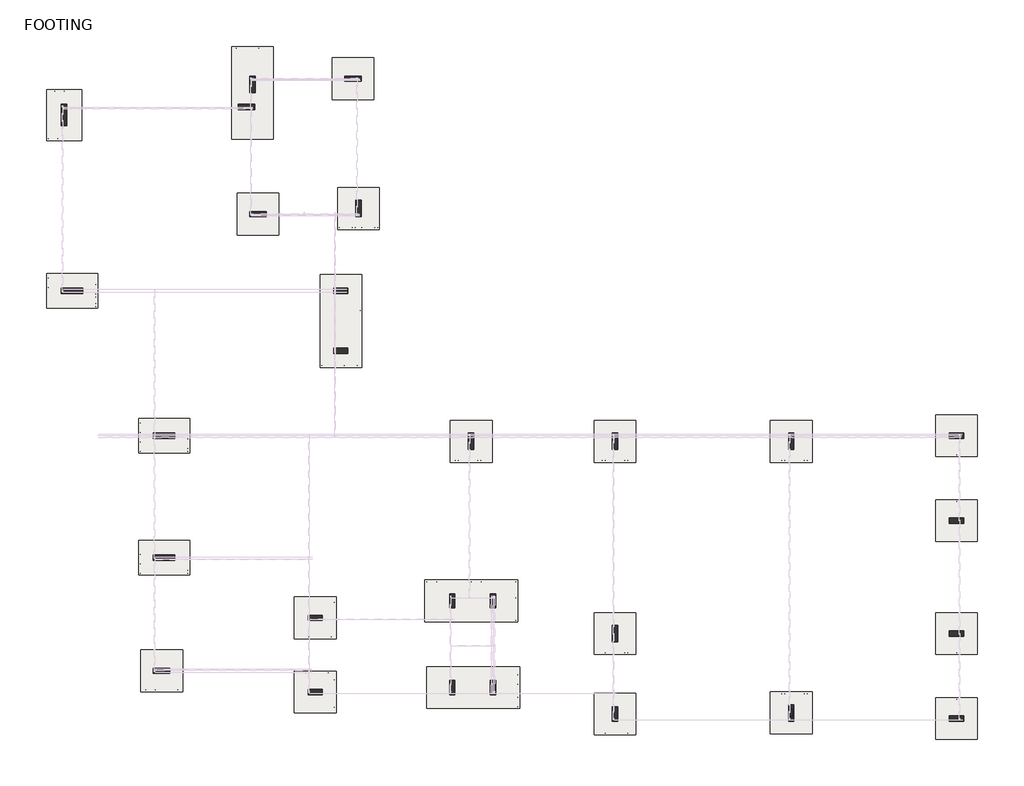
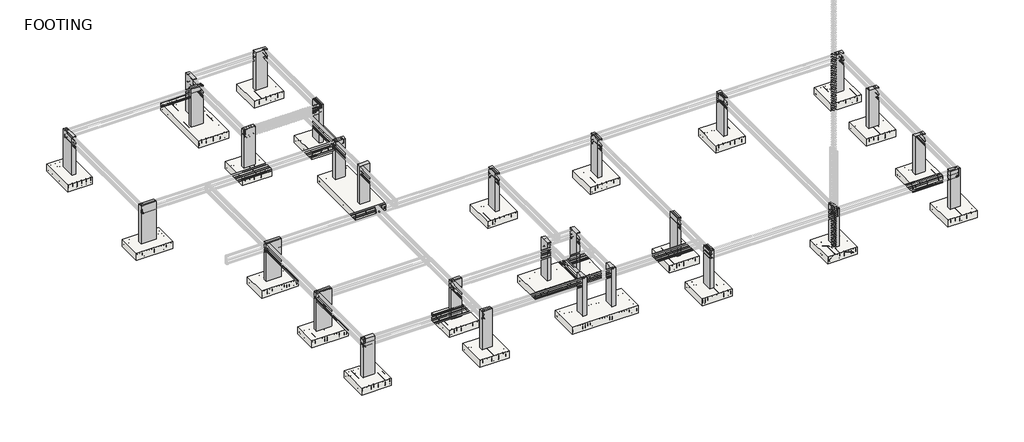
# One storey, part 1 of 12: 28 columns, 24 slabs.
"""IFC4 building model written with IfcOpenShell, lengths in millimetres."""

from ifc_helpers import new_model, si_unit, frame, origin, place, context, project, spatial, polyline, outline, extrude, faceted_brep, transform, mapped, element, save
from components import m_footing_rectangular_e5d4dde8, m_footing_rectangular_b51645d7, m_footing_rectangular_2200_x1500m_x450mm_63325679

model = new_model("IFC4")

# Units and contexts
model_context = context("Model", 3, world=origin())
ifc_project = project(units=[si_unit("LENGTHUNIT", "METRE", prefix="MILLI")], contexts=[model_context])

# Site, building, storey
site = spatial("IfcSite", under=ifc_project)
building = spatial("IfcBuilding", under=site)
storey = spatial("IfcBuildingStorey", under=building, Name="FOOTING", Elevation=-5638.8)

# Columns
placement = place(None, origin())
element("IfcColumn", 1, ObjectType="M_Concrete-Rectangular-Column : 9\" X 24\" C3", at=placement, inside=storey, context=model_context, shape_type="SweptSolid", body=[
    extrude(outline(polyline([(-8729.9501665, -13101.6041655), (-8120.3501665, -13101.6041655), (-8120.3501665, -13330.2041655), (-8729.9501665, -13330.2041655), (-8729.9501665, -13101.6041655)])), frame((0.0, 0.0, -5638.8), z_axis=(0.0, 0.0, 1.0), x_axis=(1.0, 0.0, 0.0)), (0.0, 0.0, 1.0), 2438.4),
])
element("IfcColumn", 2, ObjectType="M_Concrete-Rectangular-Column : 9\" X 24\" C3", at=placement, inside=storey, context=model_context, shape_type="SweptSolid", body=[
    extrude(outline(polyline([(-2633.9501665, -13330.2041655), (-2633.9501665, -12720.6041655), (-2405.3501665, -12720.6041655), (-2405.3501665, -13330.2041655), (-2633.9501665, -13330.2041655)])), frame((0.0, 0.0, -5638.8), z_axis=(0.0, 0.0, 1.0), x_axis=(1.0, 0.0, 0.0)), (0.0, 0.0, 1.0), 2438.4),
])
element("IfcColumn", 3, ObjectType="M_Concrete-Rectangular-Column : 9\" X 24\" C3", at=placement, inside=storey, context=model_context, shape_type="SweptSolid", body=[
    extrude(outline(polyline([(-2633.9501665, -9596.4041655), (-2633.9501665, -8986.8041655), (-2405.3501665, -8986.8041655), (-2405.3501665, -9596.4041655), (-2633.9501665, -9596.4041655)])), frame((0.0, 0.0, -5638.8), z_axis=(0.0, 0.0, 1.0), x_axis=(1.0, 0.0, 0.0)), (0.0, 0.0, 1.0), 2438.4),
])
element("IfcColumn", 4, ObjectType="M_Concrete-Rectangular-Column : 9\" X 24\" C3", at=placement, inside=storey, context=model_context, shape_type="SweptSolid", body=[
    extrude(outline(polyline([(-881.3501665, -9596.4041655), (-881.3501665, -8986.8041655), (-652.7501665, -8986.8041655), (-652.7501665, -9596.4041655), (-881.3501665, -9596.4041655)])), frame((0.0, 0.0, -5638.8), z_axis=(0.0, 0.0, 1.0), x_axis=(1.0, 0.0, 0.0)), (0.0, 0.0, 1.0), 2438.4),
])
element("IfcColumn", 5, ObjectType="M_Concrete-Rectangular-Column : 9\" X 24\" C3", at=placement, inside=storey, context=model_context, shape_type="SweptSolid", body=[
    extrude(outline(polyline([(19514.8498335, -14473.2041655), (18905.2498335, -14473.2041655), (18905.2498335, -14244.6041655), (19514.8498335, -14244.6041655), (19514.8498335, -14473.2041655)])), frame((0.0, 0.0, -5638.8), z_axis=(0.0, 0.0, 1.0), x_axis=(1.0, 0.0, 0.0)), (0.0, 0.0, 1.0), 2438.4),
])
element("IfcColumn", 6, ObjectType="M_Concrete-Rectangular-Column : 9\" X 24\" C3", at=placement, inside=storey, context=model_context, shape_type="Brep", body=[
    faceted_brep([(19514.8498335, -10815.6041655, -5638.8), (18905.2498335, -10815.6041655, -5638.8), (18905.2498335, -10587.0041655, -5638.8), (19514.8498335, -10587.0041655, -5638.8), (19514.8498335, -10815.6041655, -3200.4), (19286.2498335, -10815.6041655, -3200.4), (18905.2498335, -10815.6041655, -3200.4), (19514.8498335, -10815.6041655, -3800.4), (18905.2498335, -10587.0041655, -3200.4), (19286.2498335, -10587.0041655, -3200.4), (19514.8498335, -10587.0041655, -3200.4), (19514.8498335, -10587.0041655, -3800.4)], [[[0, 1, 2, 3]], [[4, 5, 6, 1, 0, 7]], [[6, 8, 2, 1]], [[8, 9, 10, 11, 3, 2]], [[10, 4, 7, 0, 3, 11]], [[4, 10, 9, 8, 6, 5]]]),
])
element("IfcColumn", 7, ObjectType="M_Concrete-Rectangular-Column : 9\" X 24\" C3", at=placement, inside=storey, context=model_context, shape_type="Brep", body=[
    faceted_brep([(19514.8498335, -5938.8041655, -5638.8), (18905.2498335, -5938.8041655, -5638.8), (18905.2498335, -5710.2041655, -5638.8), (19514.8498335, -5710.2041655, -5638.8), (19514.8498335, -5938.8041655, -3200.4), (19286.2498335, -5938.8041655, -3200.4), (18905.2498335, -5938.8041655, -3200.4), (19514.8498335, -5938.8041655, -3800.4), (18905.2498335, -5710.2041655, -3200.4), (19286.2498335, -5710.2041655, -3200.4), (19514.8498335, -5710.2041655, -3200.4), (19514.8498335, -5710.2041655, -3800.4)], [[[0, 1, 2, 3]], [[4, 5, 6, 1, 0, 7]], [[6, 8, 2, 1]], [[8, 9, 10, 11, 3, 2]], [[10, 4, 7, 0, 3, 11]], [[4, 10, 9, 8, 6, 5]]]),
])
element("IfcColumn", 8, ObjectType="M_Concrete-Rectangular-Column : 9\" X 24\" C3", at=placement, inside=storey, context=model_context, shape_type="SweptSolid", body=[
    extrude(outline(polyline([(19514.8498335, -2281.2041655), (18905.2498335, -2281.2041655), (18905.2498335, -2052.6041655), (19514.8498335, -2052.6041655), (19514.8498335, -2281.2041655)])), frame((0.0, 0.0, -5638.8), z_axis=(0.0, 0.0, 1.0), x_axis=(1.0, 0.0, 0.0)), (0.0, 0.0, 1.0), 2438.4),
])
element("IfcColumn", 9, ObjectType="M_Concrete-Rectangular-Column : 9\" X 24\" C3", at=placement, inside=storey, context=model_context, shape_type="SweptSolid", body=[
    extrude(outline(polyline([(-7015.4501665, 3967.1958345), (-7625.0501665, 3967.1958345), (-7625.0501665, 4195.7958345), (-7015.4501665, 4195.7958345), (-7015.4501665, 3967.1958345)])), frame((0.0, 0.0, -5638.8), z_axis=(0.0, 0.0, 1.0), x_axis=(1.0, 0.0, 0.0)), (0.0, 0.0, 1.0), 2438.4),
])
element("IfcColumn", 10, ObjectType="M_Concrete-Rectangular-Column : 9\" X 24\" C3", at=placement, inside=storey, context=model_context, shape_type="Brep", body=[
    faceted_brep([(-7015.4501665, 1376.3958345, -5638.8), (-7625.0501665, 1376.3958345, -5638.8), (-7625.0501665, 1604.9958345, -5638.8), (-7015.4501665, 1604.9958345, -5638.8), (-7015.4501665, 1376.3958345, -3200.4), (-7396.4501665, 1376.3958345, -3200.4), (-7625.0501665, 1376.3958345, -3200.4), (-7625.0501665, 1376.3958345, -3800.4), (-7625.0501665, 1604.9958345, -3200.4), (-7625.0501665, 1604.9958345, -3800.4), (-7396.4501665, 1604.9958345, -3200.4), (-7015.4501665, 1604.9958345, -3200.4)], [[[0, 1, 2, 3]], [[4, 5, 6, 7, 1, 0]], [[6, 8, 9, 2, 1, 7]], [[8, 10, 11, 3, 2, 9]], [[11, 4, 0, 3]], [[4, 11, 10, 8, 6, 5]]]),
])
element("IfcColumn", 11, ObjectType="M_Concrete-Rectangular-Column : 9\" X 24\" C3", at=placement, inside=storey, context=model_context, shape_type="SweptSolid", body=[
    extrude(outline(polyline([(-8729.9501665, -9901.2041655), (-8120.3501665, -9901.2041655), (-8120.3501665, -10129.8041655), (-8729.9501665, -10129.8041655), (-8729.9501665, -9901.2041655)])), frame((0.0, 0.0, -5638.8), z_axis=(0.0, 0.0, 1.0), x_axis=(1.0, 0.0, 0.0)), (0.0, 0.0, 1.0), 2438.4),
])
element("IfcColumn", 12, ObjectType="M_Concrete-Rectangular-Column : 9\" X 24\" C3", at=placement, inside=storey, context=model_context, shape_type="SweptSolid", body=[
    extrude(outline(polyline([(-652.7501665, -12720.6041655), (-652.7501665, -13330.2041655), (-881.3501665, -13330.2041655), (-881.3501665, -12720.6041655), (-652.7501665, -12720.6041655)])), frame((0.0, 0.0, -5638.8), z_axis=(0.0, 0.0, 1.0), x_axis=(1.0, 0.0, 0.0)), (0.0, 0.0, 1.0), 2438.4),
])
element("IfcColumn", 13, ObjectType="M_Concrete-Rectangular-Column : 9\" X 24\" C3", at=placement, inside=storey, context=model_context, shape_type="SweptSolid", body=[
    extrude(outline(polyline([(4605.0498335, -13863.6041655), (4605.0498335, -14473.2041655), (4376.4498335, -14473.2041655), (4376.4498335, -13863.6041655), (4605.0498335, -13863.6041655)])), frame((0.0, 0.0, -5638.8), z_axis=(0.0, 0.0, 1.0), x_axis=(1.0, 0.0, 0.0)), (0.0, 0.0, 1.0), 2438.4),
])
element("IfcColumn", 14, ObjectType="M_Concrete-Rectangular-Column : 9\" X 28\" C2", at=placement, inside=storey, context=model_context, shape_type="SweptSolid", body=[
    extrude(outline(polyline([(-15397.4501665, -12187.2041655), (-14686.2501665, -12187.2041655), (-14686.2501665, -12415.8041655), (-15397.4501665, -12415.8041655), (-15397.4501665, -12187.2041655)])), frame((0.0, 0.0, -5638.8), z_axis=(0.0, 0.0, 1.0), x_axis=(1.0, 0.0, 0.0)), (0.0, 0.0, 1.0), 2438.4),
])
element("IfcColumn", 15, ObjectType="M_Concrete-Rectangular-Column : 9\" X 28\" C2", at=placement, inside=storey, context=model_context, shape_type="Brep", body=[
    faceted_brep([(4376.4498335, -11056.9041655, -5638.8), (4376.4498335, -10345.7041655, -5638.8), (4605.0498335, -10345.7041655, -5638.8), (4605.0498335, -11056.9041655, -5638.8), (4376.4498335, -11056.9041655, -3200.4), (4376.4498335, -10345.7041655, -3200.4), (4376.4498335, -10345.7041655, -3800.4), (4376.4498335, -11056.9041655, -3800.4), (4605.0498335, -10345.7041655, -3200.4), (4605.0498335, -10345.7041655, -3800.4), (4605.0498335, -11056.9041655, -3200.4), (4605.0498335, -11056.9041655, -3800.4)], [[[0, 1, 2, 3]], [[4, 5, 6, 1, 0, 7]], [[5, 8, 9, 2, 1, 6]], [[8, 10, 11, 3, 2, 9]], [[10, 4, 7, 0, 3, 11]], [[4, 10, 8, 5]]]),
])
element("IfcColumn", 16, ObjectType="M_Concrete-Rectangular-Column : 9\" X 28\" C2", at=placement, inside=storey, context=model_context, shape_type="Brep", body=[
    faceted_brep([(11971.0498335, -14473.2041655, -5638.8), (11971.0498335, -13762.0041655, -5638.8), (12199.6498335, -13762.0041655, -5638.8), (12199.6498335, -14473.2041655, -5638.8), (11971.0498335, -14473.2041655, -3200.4), (11971.0498335, -14244.6041655, -3200.4), (11971.0498335, -13762.0041655, -3200.4), (11971.0498335, -14473.2041655, -3800.4), (12199.6498335, -13762.0041655, -3200.4), (12199.6498335, -14244.6041655, -3200.4), (12199.6498335, -14473.2041655, -3200.4), (12199.6498335, -14473.2041655, -3800.4)], [[[0, 1, 2, 3]], [[4, 5, 6, 1, 0, 7]], [[6, 8, 2, 1]], [[8, 9, 10, 11, 3, 2]], [[10, 4, 7, 0, 3, 11]], [[4, 10, 9, 8, 6, 5]]]),
])
element("IfcColumn", 17, ObjectType="M_Concrete-Rectangular-Column : 9\" X 28\" C2", at=placement, inside=storey, context=model_context, shape_type="Brep", body=[
    faceted_brep([(12199.6498335, -2052.6041655, -5638.8), (12199.6498335, -2763.8041655, -5638.8), (11971.0498335, -2763.8041655, -5638.8), (11971.0498335, -2052.6041655, -5638.8), (12199.6498335, -2052.6041655, -3200.4), (12199.6498335, -2281.2041655, -3200.4), (12199.6498335, -2763.8041655, -3200.4), (12199.6498335, -2052.6041655, -3800.4), (11971.0498335, -2763.8041655, -3200.4), (11971.0498335, -2281.2041655, -3200.4), (11971.0498335, -2052.6041655, -3200.4), (11971.0498335, -2052.6041655, -3800.4)], [[[0, 1, 2, 3]], [[4, 5, 6, 1, 0, 7]], [[6, 8, 2, 1]], [[8, 9, 10, 11, 3, 2]], [[10, 4, 7, 0, 3, 11]], [[4, 10, 9, 8, 6, 5]]]),
])
element("IfcColumn", 18, ObjectType="M_Concrete-Rectangular-Column : 9\" X 28\" C2", at=placement, inside=storey, context=model_context, shape_type="Brep", body=[
    faceted_brep([(4605.0498335, -2052.6041655, -5638.8), (4605.0498335, -2763.8041655, -5638.8), (4376.4498335, -2763.8041655, -5638.8), (4376.4498335, -2052.6041655, -5638.8), (4605.0498335, -2052.6041655, -3200.4), (4605.0498335, -2281.2041655, -3200.4), (4605.0498335, -2763.8041655, -3200.4), (4605.0498335, -2052.6041655, -3800.4), (4376.4498335, -2763.8041655, -3200.4), (4376.4498335, -2281.2041655, -3200.4), (4376.4498335, -2052.6041655, -3200.4), (4376.4498335, -2052.6041655, -3800.4)], [[[0, 1, 2, 3]], [[4, 5, 6, 1, 0, 7]], [[6, 8, 2, 1]], [[8, 9, 10, 11, 3, 2]], [[10, 4, 7, 0, 3, 11]], [[4, 10, 9, 8, 6, 5]]]),
])
element("IfcColumn", 19, ObjectType="M_Concrete-Rectangular-Column : 9\" X 28\" C2", at=placement, inside=storey, context=model_context, shape_type="Brep", body=[
    faceted_brep([(-1592.5501665, -2052.6041655, -5638.8), (-1592.5501665, -2763.8041655, -5638.8), (-1821.1501665, -2763.8041655, -5638.8), (-1821.1501665, -2052.6041655, -5638.8), (-1592.5501665, -2052.6041655, -3200.4), (-1592.5501665, -2281.2041655, -3200.4), (-1592.5501665, -2763.8041655, -3200.4), (-1592.5501665, -2052.6041655, -3800.4), (-1821.1501665, -2763.8041655, -3200.4), (-1821.1501665, -2281.2041655, -3200.4), (-1821.1501665, -2052.6041655, -3200.4), (-1821.1501665, -2052.6041655, -3800.4)], [[[0, 1, 2, 3]], [[4, 5, 6, 1, 0, 7]], [[6, 8, 2, 1]], [[8, 9, 10, 11, 3, 2]], [[10, 4, 7, 0, 3, 11]], [[4, 10, 9, 8, 6, 5]]]),
])
element("IfcColumn", 20, ObjectType="M_Concrete-Rectangular-Column : 9\" X 28\" C2", at=placement, inside=storey, context=model_context, shape_type="SweptSolid", body=[
    extrude(outline(polyline([(-11244.5501665, 7503.5858661), (-10533.3501665, 7503.5858661), (-10533.3501665, 7274.9858661), (-11244.5501665, 7274.9858661), (-11244.5501665, 7503.5858661)])), frame((0.0, 0.0, -5638.8), z_axis=(0.0, 0.0, 1.0), x_axis=(1.0, 0.0, 0.0)), (0.0, 0.0, 1.0), 2438.4),
])
element("IfcColumn", 21, ObjectType="M_Concrete-Rectangular-Column : 9\" X 28\" C2", at=placement, inside=storey, context=model_context, shape_type="SweptSolid", body=[
    extrude(outline(polyline([(-6672.5501665, 7274.9858661), (-6672.5501665, 7986.1858661), (-6443.9501665, 7986.1858661), (-6443.9501665, 7274.9858661), (-6672.5501665, 7274.9858661)])), frame((0.0, 0.0, -5638.8), z_axis=(0.0, 0.0, 1.0), x_axis=(1.0, 0.0, 0.0)), (0.0, 0.0, 1.0), 2438.4),
])
element("IfcColumn", 22, ObjectType="M_Concrete-Rectangular-Column : 9\" X 28\" C2", at=placement, inside=storey, context=model_context, shape_type="Brep", body=[
    faceted_brep([(-11028.6501665, 11891.9958345, -5638.8), (-11739.8501665, 11891.9958345, -5638.8), (-11739.8501665, 12120.5958345, -5638.8), (-11028.6501665, 12120.5958345, -5638.8), (-11028.6501665, 11891.9958345, -3200.4), (-11244.5501665, 11891.9958345, -3200.4), (-11739.8501665, 11891.9958345, -3200.4), (-11028.6501665, 11891.9958345, -3800.4), (-11739.8501665, 12120.5958345, -3200.4), (-11244.5501665, 12120.5958345, -3200.4), (-11028.6501665, 12120.5958345, -3200.4), (-11028.6501665, 12120.5958345, -3800.4)], [[[0, 1, 2, 3]], [[4, 5, 6, 1, 0, 7]], [[6, 8, 2, 1]], [[8, 9, 10, 11, 3, 2]], [[10, 4, 7, 0, 3, 11]], [[4, 10, 9, 8, 6, 5]]]),
])
element("IfcColumn", 23, ObjectType="M_Concrete-Rectangular-Column : 9\" X 28\" C2", at=placement, inside=storey, context=model_context, shape_type="SweptSolid", body=[
    extrude(outline(polyline([(-11015.9501665, 13339.7958345), (-11015.9501665, 12628.5958345), (-11244.5501665, 12628.5958345), (-11244.5501665, 13339.7958345), (-11015.9501665, 13339.7958345)])), frame((0.0, 0.0, -5638.8), z_axis=(0.0, 0.0, 1.0), x_axis=(1.0, 0.0, 0.0)), (0.0, 0.0, 1.0), 2438.4),
])
element("IfcColumn", 24, ObjectType="M_Concrete-Rectangular-Column : 9\" X 28\" C2", at=placement, inside=storey, context=model_context, shape_type="SweptSolid", body=[
    extrude(outline(polyline([(-7155.1501665, 13339.7958345), (-6443.9501665, 13339.7958345), (-6443.9501665, 13111.1958345), (-7155.1501665, 13111.1958345), (-7155.1501665, 13339.7958345)])), frame((0.0, 0.0, -5638.8), z_axis=(0.0, 0.0, 1.0), x_axis=(1.0, 0.0, 0.0)), (0.0, 0.0, 1.0), 2438.4),
])
element("IfcColumn", 25, ObjectType="M_Concrete-Rectangular-Column : 9\" X 36\" C1", at=placement, inside=storey, context=model_context, shape_type="SweptSolid", body=[
    extrude(outline(polyline([(-19131.2501665, 12120.5958345), (-19131.2501665, 11206.1958345), (-19359.8501665, 11206.1958345), (-19359.8501665, 12120.5958345), (-19131.2501665, 12120.5958345)])), frame((0.0, 0.0, -5638.8), z_axis=(0.0, 0.0, 1.0), x_axis=(1.0, 0.0, 0.0)), (0.0, 0.0, 1.0), 2438.4),
])
element("IfcColumn", 26, ObjectType="M_Concrete-Rectangular-Column : 9\" X 36\" C1", at=placement, inside=storey, context=model_context, shape_type="SweptSolid", body=[
    extrude(outline(polyline([(-19359.8501665, 4195.7958345), (-18445.4501665, 4195.7958345), (-18445.4501665, 3967.1958345), (-19359.8501665, 3967.1958345), (-19359.8501665, 4195.7958345)])), frame((0.0, 0.0, -5638.8), z_axis=(0.0, 0.0, 1.0), x_axis=(1.0, 0.0, 0.0)), (0.0, 0.0, 1.0), 2438.4),
])
element("IfcColumn", 27, ObjectType="M_Concrete-Rectangular-Column : 9\" X 36\" C1", at=placement, inside=storey, context=model_context, shape_type="Brep", body=[
    faceted_brep([(-15397.4501665, -2052.6041655, -5638.8), (-14483.0501665, -2052.6041655, -5638.8), (-14483.0501665, -2281.2041655, -5638.8), (-15397.4501665, -2281.2041655, -5638.8), (-15397.4501665, -2052.6041655, -3200.4), (-14483.0501665, -2052.6041655, -3200.4), (-14483.0501665, -2281.2041655, -3200.4), (-15168.8501665, -2281.2041655, -3200.4), (-15397.4501665, -2281.2041655, -3200.4), (-15397.4501665, -2281.2041655, -3800.4)], [[[0, 1, 2, 3]], [[4, 5, 1, 0]], [[5, 6, 2, 1]], [[6, 7, 8, 9, 3, 2]], [[8, 4, 0, 3, 9]], [[4, 8, 7, 6, 5]]]),
])
element("IfcColumn", 28, ObjectType="M_Concrete-Rectangular-Column : 9\" X 36\" C1", at=placement, inside=storey, context=model_context, shape_type="Brep", body=[
    faceted_brep([(-15397.4501665, -7310.4041655, -5638.8), (-14483.0501665, -7310.4041655, -5638.8), (-14483.0501665, -7539.0041655, -5638.8), (-15397.4501665, -7539.0041655, -5638.8), (-15397.4501665, -7310.4041655, -3200.4), (-15168.8501665, -7310.4041655, -3200.4), (-14483.0501665, -7310.4041655, -3200.4), (-15397.4501665, -7310.4041655, -3800.4), (-14483.0501665, -7539.0041655, -3200.4), (-15168.8501665, -7539.0041655, -3200.4), (-15397.4501665, -7539.0041655, -3200.4), (-15397.4501665, -7539.0041655, -3800.4)], [[[0, 1, 2, 3]], [[4, 5, 6, 1, 0, 7]], [[6, 8, 2, 1]], [[8, 9, 10, 11, 3, 2]], [[10, 4, 7, 0, 3, 11]], [[4, 10, 9, 8, 6, 5]]]),
])

# Slabs
m_footing_rectangular_shape = m_footing_rectangular_e5d4dde8(model_context)
element("IfcSlab", 29, ObjectType="M_Footing-Rectangular", at=placement, inside=storey, context=model_context, shape_type="MappedRepresentation", body=[
    mapped(m_footing_rectangular_shape, transform((19210.0498335, -14358.9041655, -5638.8), x_axis=(1.0, 0.0, 0.0), y_axis=(0.0, 1.0, 0.0), z_axis=(0.0, 0.0, 1.0))),
])
element("IfcSlab", 30, ObjectType="M_Footing-Rectangular", at=placement, inside=storey, context=model_context, shape_type="MappedRepresentation", body=[
    mapped(m_footing_rectangular_shape, transform((19210.0498335, -10701.3041655, -5638.8), x_axis=(1.0, 0.0, 0.0), y_axis=(0.0, 1.0, 0.0), z_axis=(0.0, 0.0, 1.0))),
])
element("IfcSlab", 31, ObjectType="M_Footing-Rectangular", at=placement, inside=storey, context=model_context, shape_type="MappedRepresentation", body=[
    mapped(m_footing_rectangular_shape, transform((19210.0498335, -5824.5041655, -5638.8), x_axis=(1.0, 0.0, 0.0), y_axis=(0.0, 1.0, 0.0), z_axis=(0.0, 0.0, 1.0))),
])
element("IfcSlab", 32, ObjectType="M_Footing-Rectangular", at=placement, inside=storey, context=model_context, shape_type="MappedRepresentation", body=[
    mapped(m_footing_rectangular_shape, transform((19210.0498335, -2166.9041655, -5638.8), x_axis=(1.0, 0.0, 0.0), y_axis=(0.0, 1.0, 0.0), z_axis=(0.0, 0.0, 1.0))),
])
element("IfcSlab", 33, ObjectType="M_Footing-Rectangular", at=placement, inside=storey, context=model_context, shape_type="MappedRepresentation", body=[
    mapped(m_footing_rectangular_shape, transform((12085.3498335, -2408.2041655, -5638.8), x_axis=(1.0, 0.0, 0.0), y_axis=(0.0, 1.0, 0.0), z_axis=(0.0, 0.0, 1.0))),
])
element("IfcSlab", 34, ObjectType="M_Footing-Rectangular", at=placement, inside=storey, context=model_context, shape_type="MappedRepresentation", body=[
    mapped(m_footing_rectangular_shape, transform((12085.3498335, -14117.6041655, -5638.8), x_axis=(1.0, 0.0, 0.0), y_axis=(0.0, 1.0, 0.0), z_axis=(0.0, 0.0, 1.0))),
])
element("IfcSlab", 35, ObjectType="M_Footing-Rectangular", at=placement, inside=storey, context=model_context, shape_type="MappedRepresentation", body=[
    mapped(m_footing_rectangular_shape, transform((4490.7498335, -2408.2041655, -5638.8), x_axis=(1.0, 0.0, 0.0), y_axis=(0.0, 1.0, 0.0), z_axis=(0.0, 0.0, 1.0))),
])
element("IfcSlab", 36, ObjectType="M_Footing-Rectangular", at=placement, inside=storey, context=model_context, shape_type="MappedRepresentation", body=[
    mapped(m_footing_rectangular_shape, transform((4490.7498335, -14168.4041655, -5638.8), x_axis=(1.0, 0.0, 0.0), y_axis=(0.0, 1.0, 0.0), z_axis=(0.0, 0.0, 1.0))),
])
element("IfcSlab", 37, ObjectType="M_Footing-Rectangular", at=placement, inside=storey, context=model_context, shape_type="MappedRepresentation", body=[
    mapped(m_footing_rectangular_shape, transform((4490.7498335, -10701.3041655, -5638.8), x_axis=(1.0, 0.0, 0.0), y_axis=(0.0, 1.0, 0.0), z_axis=(0.0, 0.0, 1.0))),
])
element("IfcSlab", 38, ObjectType="M_Footing-Rectangular", at=placement, inside=storey, context=model_context, shape_type="MappedRepresentation", body=[
    mapped(m_footing_rectangular_shape, transform((-8425.1501665, -13215.9041655, -5638.8), x_axis=(1.0, 0.0, 0.0), y_axis=(0.0, 1.0, 0.0), z_axis=(0.0, 0.0, 1.0))),
])
element("IfcSlab", 39, ObjectType="M_Footing-Rectangular", at=placement, inside=storey, context=model_context, shape_type="MappedRepresentation", body=[
    mapped(m_footing_rectangular_shape, transform((-8425.1501665, -10015.5041655, -5638.8), x_axis=(1.0, 0.0, 0.0), y_axis=(0.0, 1.0, 0.0), z_axis=(0.0, 0.0, 1.0))),
])
element("IfcSlab", 40, ObjectType="M_Footing-Rectangular", at=placement, inside=storey, context=model_context, shape_type="MappedRepresentation", body=[
    mapped(m_footing_rectangular_shape, transform((-15041.8501665, -12301.5041655, -5638.8), x_axis=(1.0, 0.0, 0.0), y_axis=(0.0, 1.0, 0.0), z_axis=(0.0, 0.0, 1.0))),
])
element("IfcSlab", 41, ObjectType="M_Footing-Rectangular", at=placement, inside=storey, context=model_context, shape_type="MappedRepresentation", body=[
    mapped(m_footing_rectangular_shape, transform((-6799.5501665, 13225.4958345, -5638.8), x_axis=(1.0, 0.0, 0.0), y_axis=(0.0, 1.0, 0.0), z_axis=(0.0, 0.0, 1.0))),
])
element("IfcSlab", 42, ObjectType="M_Footing-Rectangular", at=placement, inside=storey, context=model_context, shape_type="MappedRepresentation", body=[
    mapped(m_footing_rectangular_shape, transform((-10888.9501665, 7389.2858661, -5638.8), x_axis=(1.0, 0.0, 0.0), y_axis=(0.0, 1.0, 0.0), z_axis=(0.0, 0.0, 1.0))),
])
element("IfcSlab", 43, ObjectType="M_Footing-Rectangular", at=placement, inside=storey, context=model_context, shape_type="MappedRepresentation", body=[
    mapped(m_footing_rectangular_shape, transform((-6558.2501665, 7630.5858661, -5638.8), x_axis=(1.0, 0.0, 0.0), y_axis=(0.0, 1.0, 0.0), z_axis=(0.0, 0.0, 1.0))),
])
element("IfcSlab", 44, ObjectType="M_Footing-Rectangular", at=placement, inside=storey, context=model_context, shape_type="MappedRepresentation", body=[
    mapped(m_footing_rectangular_shape, transform((-1706.8501665, -2408.2041655, -5638.8), x_axis=(1.0, 0.0, 0.0), y_axis=(0.0, 1.0, 0.0), z_axis=(0.0, 0.0, 1.0))),
])
m_footing_rectangular_2_shape = m_footing_rectangular_b51645d7(model_context)
element("IfcSlab", 45, ObjectType="M_Footing-Rectangular", at=placement, inside=storey, context=model_context, shape_type="MappedRepresentation", body=[
    mapped(m_footing_rectangular_2_shape, transform((-1619.6501665, -13025.4041655, -5638.8), x_axis=(0.0, 1.0, 0.0), y_axis=(-1.0, 0.0, 0.0), z_axis=(0.0, 0.0, 1.0))),
])
element("IfcSlab", 46, ObjectType="M_Footing-Rectangular", at=placement, inside=storey, context=model_context, shape_type="MappedRepresentation", body=[
    mapped(m_footing_rectangular_2_shape, transform((-1706.8501665, -9291.6041655, -5638.8), x_axis=(0.0, 1.0, 0.0), y_axis=(-1.0, 0.0, 0.0), z_axis=(0.0, 0.0, 1.0))),
])
element("IfcSlab", 47, ObjectType="M_Footing-Rectangular", at=placement, inside=storey, context=model_context, shape_type="MappedRepresentation", body=[
    mapped(m_footing_rectangular_2_shape, transform((-7310.7501665, 2781.4958345, -5638.8), x_axis=(1.0, 0.0, 0.0), y_axis=(0.0, 1.0, 0.0), z_axis=(0.0, 0.0, 1.0))),
])
element("IfcSlab", 48, ObjectType="M_Footing-Rectangular", at=placement, inside=storey, context=model_context, shape_type="MappedRepresentation", body=[
    mapped(m_footing_rectangular_2_shape, transform((-11130.2501665, 12615.9958345, -5638.8), x_axis=(1.0, 0.0, 0.0), y_axis=(0.0, 1.0, 0.0), z_axis=(0.0, 0.0, 1.0))),
])
m_footing_rectangular_2200_x1500m_x450mm_shape = m_footing_rectangular_2200_x1500m_x450mm_63325679(model_context)
element("IfcSlab", 49, ObjectType="M_Footing-Rectangular : 2200 X1500M X450MM", at=placement, inside=storey, context=model_context, shape_type="MappedRepresentation", body=[
    mapped(m_footing_rectangular_2200_x1500m_x450mm_shape, transform((-19245.5501665, 11663.3958345, -5638.8), x_axis=(1.0, 0.0, 0.0), y_axis=(0.0, 1.0, 0.0), z_axis=(0.0, 0.0, 1.0))),
])
element("IfcSlab", 50, ObjectType="M_Footing-Rectangular : 2200 X1500M X450MM", at=placement, inside=storey, context=model_context, shape_type="MappedRepresentation", body=[
    mapped(m_footing_rectangular_2200_x1500m_x450mm_shape, transform((-18902.6501665, 4081.4958345, -5638.8), x_axis=(0.0, 1.0, 0.0), y_axis=(-1.0, 0.0, 0.0), z_axis=(0.0, 0.0, 1.0))),
])
element("IfcSlab", 51, ObjectType="M_Footing-Rectangular : 2200 X1500M X450MM", at=placement, inside=storey, context=model_context, shape_type="MappedRepresentation", body=[
    mapped(m_footing_rectangular_2200_x1500m_x450mm_shape, transform((-14940.2501665, -2166.9041655, -5638.8), x_axis=(0.0, 1.0, 0.0), y_axis=(-1.0, 0.0, 0.0), z_axis=(0.0, 0.0, 1.0))),
])
element("IfcSlab", 52, ObjectType="M_Footing-Rectangular : 2200 X1500M X450MM", at=placement, inside=storey, context=model_context, shape_type="MappedRepresentation", body=[
    mapped(m_footing_rectangular_2200_x1500m_x450mm_shape, transform((-14940.2501665, -7424.7041655, -5638.8), x_axis=(0.0, 1.0, 0.0), y_axis=(-1.0, 0.0, 0.0), z_axis=(0.0, 0.0, 1.0))),
])

save(model, "model.ifc")

# Revit data of these elements
# Grids (mm)
#   "10": line (-20856.059, 12006.296) -> (-4734.26, 12006.296)
#   "L": line (-6558.25, 312.467) -> (-6558.25, 15849.853)
#   "K": line (-11130.25, 312.467) -> (-11130.25, 15849.853)
#   "A": line (-15283.15, -827.926) -> (-15283.15, -17253.076)
#   "J": line (-19245.55, 312.467) -> (-19245.55, 15849.853)
#   "a": line (-8615.65, -5050.347) -> (-8615.65, -15986.845)
#   "E": line (-1706.85, -6410.26) -> (-1706.85, -827.926)
#   "M": line (-7510.75, 5465.974) -> (-7510.75, 312.467)
#   "3": line (23091.477, -10701.304) -> (-18188.7, -10701.304)
#   "5": line (-18188.7, -5824.504) -> (23091.477, -5824.504)
#   "7": line (-4734.26, 1490.696) -> (-20856.059, 1490.696)
#   "8": line (-4734.26, 4081.496) -> (-20856.059, 4081.496)
#   "9": line (-4734.26, 7389.286) -> (-20856.059, 7389.286)
#   "11": line (-20856.059, 13225.496) -> (-4734.26, 13225.496)
#   "1": line (23091.477, -14358.904) -> (-18188.7, -14358.904)
#   "D": line (19400.55, -827.926) -> (19400.55, -17253.076)
#   "6": line (-18188.7, -2166.904) -> (23091.477, -2166.904)
#   "C": line (12085.35, -827.926) -> (12085.35, -17253.076)
#   "B": line (4490.75, -17253.076) -> (4490.75, -827.926)
#   "c": line (-767.05, -5050.347) -> (-767.05, -15986.845)
#   "b": line (-2519.65, -5050.347) -> (-2519.65, -15986.845)
#   "x": line (-10328.601, -13215.904) -> (2270.965, -13215.904)
#   "2": line (-6518.92, -12301.504) -> (-18188.7, -12301.504)
#   "4": line (-6518.92, -7424.704) -> (-18188.7, -7424.704)
#   "z": line (1110.054, -9101.104) -> (-9074.668, -9101.104)
# Type "M_Concrete-Rectangular-Column : 9\" X 24\" C3"
#   b = 228.6 mm
#   h = 609.6 mm
#   Structural Material [instance default] = Concrete, Cast-in-Place gray
# Type "M_Concrete-Rectangular-Column : 9\" X 28\" C2"
#   b = 228.6 mm
#   h = 711.2 mm
#   Structural Material [instance default] = Concrete, Cast-in-Place gray
# Type "M_Concrete-Rectangular-Column : 9\" X 36\" C1"
#   b = 228.6 mm
#   h = 914.4 mm
#   Structural Material [instance default] = Concrete, Cast-in-Place gray
# Type "M_Footing-Rectangular"
#   Width = 1800 mm
#   Length = 1800 mm
#   Foundation Thickness = 450 mm
#   Structural Material [instance default] = Concrete, Cast-in-Place gray
#   Assembly Code = ""
# Type "M_Footing-Rectangular"
#   Width = 1800 mm
#   Length = 4000 mm
#   Foundation Thickness = 450 mm
#   Structural Material [instance default] = Concrete, Cast-in-Place gray
#   Assembly Code = ""
# Type "M_Footing-Rectangular : 2200 X1500M X450MM"
#   Width = 1500 mm
#   Length = 2200 mm
#   Foundation Thickness = 450 mm
#   Structural Material [instance default] = Concrete, Cast-in-Place gray
#   Assembly Code = ""
# Elements 1, 2, 3, 4, 5, 6, 7, 8, 9, 10, 11, 12, 13 (IfcColumn, "M_Concrete-Rectangular-Column : 9\" X 24\" C3")
#   Structural Material = Concrete, Cast-in-Place gray
#   Phase Created = New Construction
#   Materials on its faces: "Concrete, Cast-in-Place gray"
# Elements 14, 15, 16, 17, 18, 19, 20, 21, 22, 23, 24 (IfcColumn, "M_Concrete-Rectangular-Column : 9\" X 28\" C2")
#   Structural Material = Concrete, Cast-in-Place gray
#   Phase Created = New Construction
#   Materials on its faces: "Concrete, Cast-in-Place gray"
# Elements 25, 26, 27, 28 (IfcColumn, "M_Concrete-Rectangular-Column : 9\" X 36\" C1")
#   Structural Material = Concrete, Cast-in-Place gray
#   Phase Created = New Construction
#   Materials on its faces: "Concrete, Cast-in-Place gray"
# Elements 29, 30, 31, 32, 33, 34, 35, 36, 37, 38, 39, 40, 41, 42, 43, 44, 45, 46, 47, 48 (IfcSlab, "M_Footing-Rectangular")
#   Structural Material = Concrete, Cast-in-Place gray
#   Phase Created = New Construction
#   Materials on its faces: "Concrete, Cast-in-Place gray"
# Elements 49, 50, 51, 52 (IfcSlab, "M_Footing-Rectangular : 2200 X1500M X450MM")
#   Structural Material = Concrete, Cast-in-Place gray
#   Phase Created = New Construction
#   Materials on its faces: "Concrete, Cast-in-Place gray"
# Materials
#   "Concrete, Cast-in-Place gray": class "Concrete", colour RGB 192 192 192, transparency 0, Description = "Cast-in-place concrete", Cost = 0
